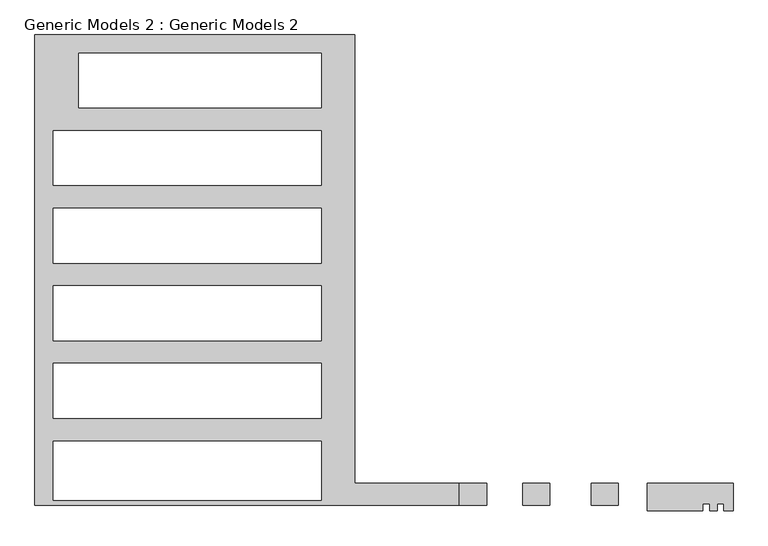
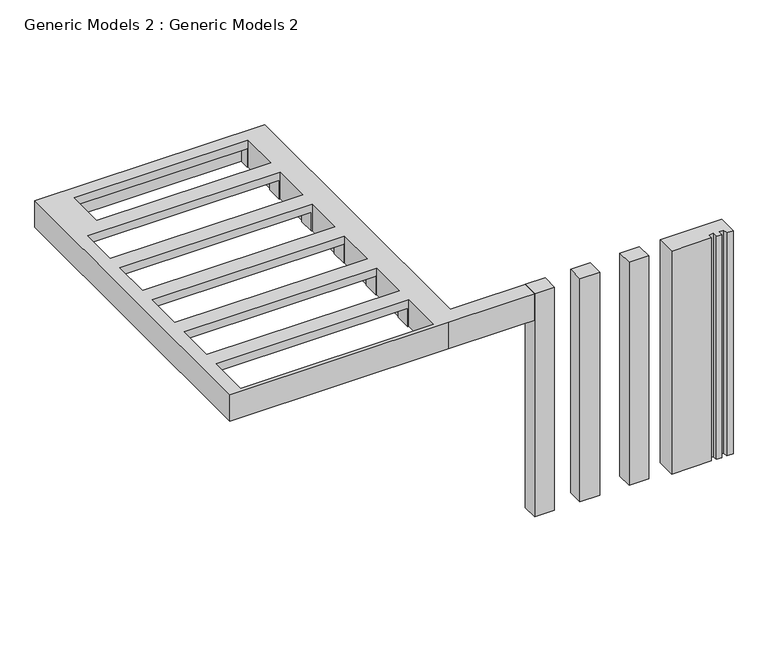
"""IFC4 building model written with IfcOpenShell, lengths in millimetres: proxy geometry, Generic Models 2 : Generic Models 2."""

from ifc_helpers import new_model, si_unit, frame, origin, place, context, project, spatial, polyline, outline, extrude, faceted_brep, source, transform, mapped, element, save


def generic_models_2_generic_models_2_13626f08(model_context):
    return source(origin(), model_context, "Body", "SolidModel", [
        extrude(outline(polyline([(-1120.3115419, -3296.2867893), (-165.4525595, -3296.2867893), (-165.4525595, -3601.0867893), (-267.5358675, -3601.0867893), (-267.5358675, -3524.8867893), (-343.7358675, -3524.8867893), (-343.7358675, -3601.0867893), (-426.2858675, -3601.0867893), (-426.2858675, -3524.8867893), (-502.4858675, -3524.8867893), (-502.4858675, -3601.0867893), (-1120.3115419, -3601.0867893), (-1120.3115419, -3296.2867893)])), frame((0.0, 0.0, 3200.4), z_axis=(0.0, 0.0, 1.0), x_axis=(1.0, 0.0, 0.0)), (0.0, 0.0, 1.0), 3657.6),
        extrude(outline(polyline([(-2203.8025595, -3543.9367893), (-2508.6025595, -3543.9367893), (-2508.6025595, -3296.2867893), (-2203.8025595, -3296.2867893), (-2203.8025595, -3543.9367893)])), frame((0.0, 0.0, 3200.4), z_axis=(0.0, 0.0, 1.0), x_axis=(1.0, 0.0, 0.0)), (0.0, 0.0, 1.0), 3657.6),
        extrude(outline(polyline([(-2906.3946608, -3543.9367893), (-3211.1946608, -3543.9367893), (-3211.1946608, -3296.2867893), (-2906.3946608, -3296.2867893), (-2906.3946608, -3543.9367893)])), frame((0.0, 0.0, 3200.4), z_axis=(0.0, 0.0, 1.0), x_axis=(1.0, 0.0, 0.0)), (0.0, 0.0, 1.0), 3657.6),
        extrude(outline(polyline([(-1441.8025595, -3543.9367893), (-1746.6025595, -3543.9367893), (-1746.6025595, -3296.2867893), (-1441.8025595, -3296.2867893), (-1441.8025595, -3543.9367893)])), frame((0.0, 0.0, 3200.4), z_axis=(0.0, 0.0, 1.0), x_axis=(1.0, 0.0, 0.0)), (0.0, 0.0, 1.0), 3657.6),
        faceted_brep([(-4375.5025595, 1694.8132107, 6858.0), (-7937.8525595, 1694.8132107, 6858.0), (-7937.8525595, -3543.9367893, 6858.0), (-4546.9525595, -3543.9367893, 6858.0), (-2906.3946608, -3543.9367893, 6858.0), (-2906.3946608, -3296.2867893, 6858.0), (-4375.5025595, -3296.2867893, 6858.0), (-4750.1525595, 1491.6132107, 6858.0), (-4750.1525595, 882.0132107, 6858.0), (-7448.554535, 882.0132107, 6858.0), (-7448.554535, 1491.6132107, 6858.0), (-7734.6525595, -2826.3867893, 6858.0), (-4750.1525595, -2826.3867893, 6858.0), (-4750.1525595, -3486.821015, 6858.0), (-7734.6525595, -3486.821015, 6858.0), (-7734.6525595, 628.0132107, 6858.0), (-4750.1525595, 628.0132107, 6858.0), (-4750.1525595, 18.4132107, 6858.0), (-7734.6525595, 18.4132107, 6858.0), (-7734.6525595, -235.5867893, 6858.0), (-4750.1525595, -235.5867893, 6858.0), (-4750.1525595, -845.1867893, 6858.0), (-7734.6525595, -845.1867893, 6858.0), (-7734.6525595, -1099.1867893, 6858.0), (-4750.1525595, -1099.1867893, 6858.0), (-4750.1525595, -1708.7867893, 6858.0), (-7734.6525595, -1708.7867893, 6858.0), (-7734.6525595, -1962.7867893, 6858.0), (-4750.1525595, -1962.7867893, 6858.0), (-4750.1525595, -2572.3867893, 6858.0), (-7734.6525595, -2572.3867893, 6858.0), (-4375.5025595, 1694.8132107, 6423.0), (-4375.5025595, -3296.2867893, 6423.0), (-2906.3946608, -3296.2867893, 6423.0), (-2906.3946608, -3543.9367893, 6423.0), (-4546.9525595, -3543.9367893, 6423.0), (-7937.8525595, -3543.9367893, 6423.0), (-7937.8525595, 1694.8132107, 6423.0), (-4750.1525595, 882.0132107, 6423.0), (-4750.1525595, 1491.6132107, 6423.0), (-4762.8525595, 1491.6132107, 6423.0), (-4762.8525595, 1643.978985, 6423.0), (-7734.6525595, 1643.978985, 6423.0), (-7734.6525595, -3486.821015, 6423.0), (-4762.8525595, -3486.821015, 6423.0), (-4750.1525595, -3486.821015, 6423.0), (-4750.1525595, -2826.3867893, 6423.0), (-4762.8525595, -2826.3867893, 6423.0), (-4762.8525595, -2572.3867893, 6423.0), (-4750.1525595, -2572.3867893, 6423.0), (-4750.1525595, -1962.7867893, 6423.0), (-4762.8525595, -1962.7867893, 6423.0), (-4762.8525595, -1708.7867893, 6423.0), (-4750.1525595, -1708.7867893, 6423.0), (-4750.1525595, -1099.1867893, 6423.0), (-4762.8525595, -1099.1867893, 6423.0), (-4762.8525595, -845.1867893, 6423.0), (-4750.1525595, -845.1867893, 6423.0), (-4750.1525595, -235.5867893, 6423.0), (-4762.8525595, -235.5867893, 6423.0), (-4762.8525595, 18.4132107, 6423.0), (-4750.1525595, 18.4132107, 6423.0), (-4750.1525595, 628.0132107, 6423.0), (-4762.8525595, 628.0132107, 6423.0), (-4762.8525595, 882.0132107, 6423.0), (-4762.8525595, 882.0132107, 6727.8), (-7448.554535, 882.0132107, 6727.8), (-7448.554535, 1491.6132107, 6727.8), (-4762.8525595, 1491.6132107, 6727.8), (-7734.6525595, -2826.3867893, 6727.8), (-4762.8525595, -2826.3867893, 6727.8), (-7734.6525595, 1643.978985, 6727.8), (-7734.6525595, 628.0132107, 6727.8), (-7734.6525595, 18.4132107, 6727.8), (-7734.6525595, -235.5867893, 6727.8), (-7734.6525595, -845.1867893, 6727.8), (-7734.6525595, -1099.1867893, 6727.8), (-7734.6525595, -1708.7867893, 6727.8), (-7734.6525595, -1962.7867893, 6727.8), (-7734.6525595, -2572.3867893, 6727.8), (-4762.8525595, 628.0132107, 6727.8), (-4762.8525595, 18.4132107, 6727.8), (-4762.8525595, -235.5867893, 6727.8), (-4762.8525595, -845.1867893, 6727.8), (-4762.8525595, -1099.1867893, 6727.8), (-4762.8525595, -1708.7867893, 6727.8), (-4762.8525595, -1962.7867893, 6727.8), (-4762.8525595, -2572.3867893, 6727.8), (-4762.8525595, 1643.978985, 6727.8)], [[[0, 1, 2, 3, 4, 5, 6], [7, 8, 9, 10], [11, 12, 13, 14], [15, 16, 17, 18], [19, 20, 21, 22], [23, 24, 25, 26], [27, 28, 29, 30]], [[31, 32, 33, 34, 35, 36, 37], [38, 39, 40, 41, 42, 43, 44, 45, 46, 47, 48, 49, 50, 51, 52, 53, 54, 55, 56, 57, 58, 59, 60, 61, 62, 63, 64]], [[1, 0, 31, 37]], [[2, 1, 37, 36]], [[3, 2, 36, 35]], [[0, 6, 32, 31]], [[8, 7, 39, 38]], [[9, 8, 38, 64, 65, 66]], [[10, 9, 66, 67]], [[7, 10, 67, 68, 40, 39]], [[12, 11, 69, 70, 47, 46]], [[13, 12, 46, 45]], [[43, 14, 13, 45, 44]], [[11, 14, 43, 42, 71, 72, 15, 18, 73, 74, 19, 22, 75, 76, 23, 26, 77, 78, 27, 30, 79, 69]], [[16, 15, 72, 80, 63, 62]], [[17, 16, 62, 61]], [[18, 17, 61, 60, 81, 73]], [[20, 19, 74, 82, 59, 58]], [[21, 20, 58, 57]], [[22, 21, 57, 56, 83, 75]], [[24, 23, 76, 84, 55, 54]], [[25, 24, 54, 53]], [[26, 25, 53, 52, 85, 77]], [[28, 27, 78, 86, 51, 50]], [[29, 28, 50, 49]], [[30, 29, 49, 48, 87, 79]], [[71, 88, 68, 67, 66, 65, 80, 72]], [[74, 73, 81, 82]], [[76, 75, 83, 84]], [[78, 77, 85, 86]], [[69, 79, 87, 70]], [[68, 88, 41, 40]], [[80, 65, 64, 63]], [[82, 81, 60, 59]], [[84, 83, 56, 55]], [[86, 85, 52, 51]], [[70, 87, 48, 47]], [[88, 71, 42, 41]], [[4, 3, 35, 34]], [[5, 4, 34, 33]], [[6, 5, 33, 32]]]),
    ])


if __name__ == "__main__":
    model = new_model("IFC4")
    model_context = context("Model", 3, world=origin())
    ifc_project = project(units=[si_unit("LENGTHUNIT", "METRE", prefix="MILLI")], contexts=[model_context])
    site = spatial("IfcSite", under=ifc_project)
    building = spatial("IfcBuilding", under=site)
    placement = place(None, origin())
    generic_models_2_generic_models_2_shape = generic_models_2_generic_models_2_13626f08(model_context)
    element("IfcBuildingElementProxy", 1, Name="Generic Models 2 : Generic Models 2", ObjectType="Generic Models 2 : Generic Models 2", at=placement, inside=building, context=model_context, shape_type="MappedRepresentation", body=[
        mapped(generic_models_2_generic_models_2_shape, transform((0.0, 0.0, 0.0), x_axis=(1.0, 0.0, 0.0), y_axis=(0.0, 1.0, 0.0), z_axis=(0.0, 0.0, 1.0))),
    ])
    save(model, "model.ifc")
